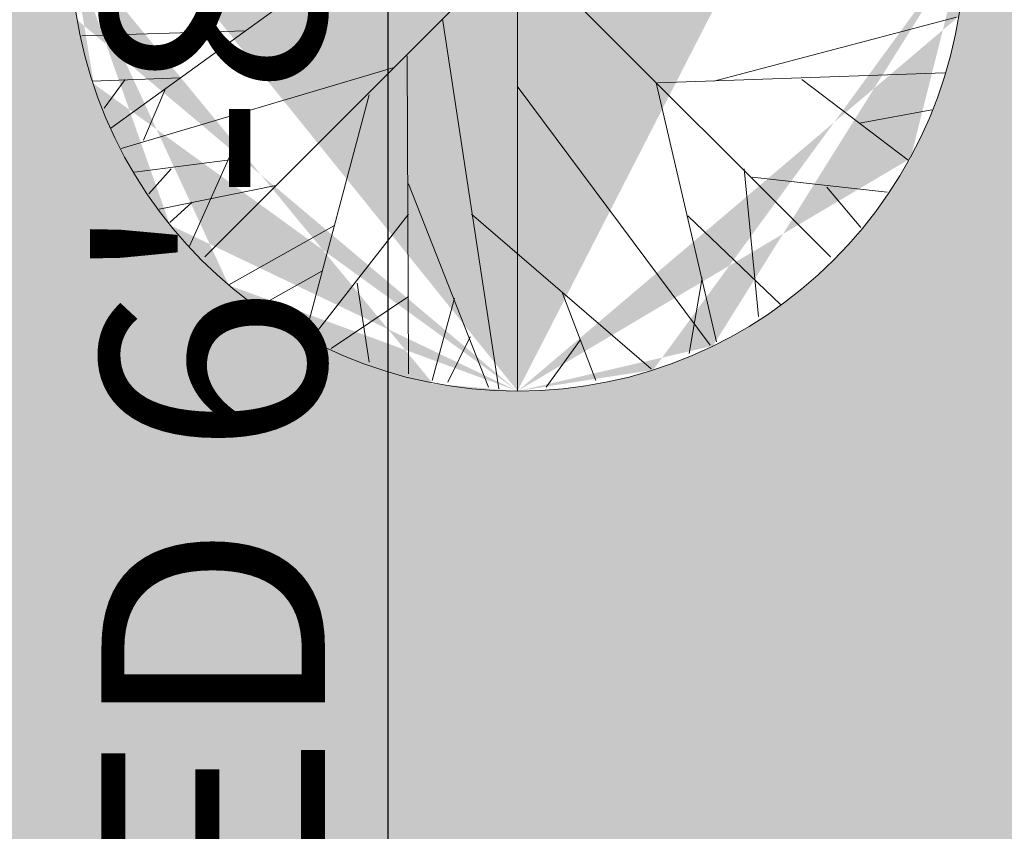
# Model space of a CAD drawing. Units: inches. Extents: x 459864 to 460310, y 324185 to 324787.
# Tile 59 of 112: x 460127 to 460154, y 324239 to 324260. Entities that reach past the tile are written whole.
import ezdxf

# ---------------------------------------------------------------- set-up
doc = ezdxf.new("R2010")
doc.units = ezdxf.units.IN
for name, color, linetype, lineweight in [('A-ANNO-DIMS', 2, 'Continuous', 18), ('L-PLNT', 3, 'Continuous', 13), ('L-SITE-PATT', 252, 'Continuous', 13)]:
    doc.layers.add(name, color=color, linetype=linetype, lineweight=lineweight)
doc.styles.get("Standard").update_dxf_attribs({"font": 'arial.ttf'})
doc.dimstyles.new('ISO-25', dxfattribs={"dimtxt": 6, "dimasz": 2.5, "dimexe": 1.25, "dimexo": 0.625, "dimtad": 1, "dimdec": 1, "dimlunit": 3, "dimtxsty": 'Standard', "dimcen": 2.5, "dimadec": 0, "dimazin": 0, "dimtfac": 1, "dimtdec": 1, "dimtmove": 0, "dimatfit": 3, "dimfxl": 1, "dimarcsym": 0})

# ---------------------------------------------------------------- blocks, each defined once
blk = doc.blocks.new('Tree - deciduous plan')
for p, q in [((0, 59.9996), (0, -60)), ((42, 42), (-42, -42)), ((42, -42), (-42, 42)), ((-54.6162, -24.7335), (-20.2853, 0.0941)), ((-10.074, -10.0627), (-2.5036, -59.7178)), ((26.3697, -18.4138), (58.9401, -9.8369)), ((-58.4895, -12.3197), (-36.4825, -11.6426)), ((-14.8275, -15.0282), (-14.6515, -57.6865)), ((-53.2078, -27.442), (-16.7641, -16.6081)), ((-57.081, -18.4138), (-45.2853, -17.9624)), ((-52.6797, -18.188), (-55.4966, -22.0251)), ((18.7992, -18.6394), (57.3556, -17.2853)), ((38.1654, -18.188), (52.426, -29.0219)), ((-47.2219, -19.3166), (-50.2148, -26.3135)), ((-0.0388, -19.0909), (25.8415, -53.8495)), ((18.6232, -18.6394), (26.7218, -53.3981)), ((-19.9331, -20.2194), (-28.5599, -52.721)), ((45.9119, -24.0564), (55.595, -22.2508)), ((-35.9543, -22.4765), (-44.0529, -40.5329)), ((-38.9472, -29.0219), (-51.4472, -30.6018)), ((-46.5177, -30.1504), (-49.5106, -33.536)), ((30.419, -30.1504), (32.3556, -50.0125)), ((31.4753, -31.279), (49.6091, -33.3103)), ((-32.4331, -32.4075), (-48.1021, -35.5674)), ((-14.6515, -32.1818), (-3.912, -59.4922)), ((41.5105, -32.6332), (46.088, -38.0501)), ((-43.7008, -34.6645), (-46.6937, -37.373)), ((-14.6515, -36.2445), (-27.6797, -52.9467)), ((-6.2008, -36.2445), (17.919, -57.0094)), ((22.8485, -36.4702), (35.3485, -48.4326)), ((-24.6867, -37.8244), (-38.7712, -45.7241)), ((-26.2712, -43.9185), (-34.7219, -48.6583)), ((24.7852, -44.8213), (23.0246, -54.978)), ((-21.5177, -45.4984), (-19.9331, -56.1065)), ((-14.6515, -47.3041), (-25.0388, -54.3009)), ((-8.4895, -47.5298), (-11.4825, -58.5893)), ((5.9471, -46.6269), (10.5246, -58.5893)), ((-6.3768, -52.721), (-9.3698, -58.815)), ((8.4119, -53.1724), (3.8344, -59.4922))]:
    blk.add_line(p, q)
blk.add_circle((0, 0), 60)
blk = doc.blocks.new('*D28')
at = {"layer": 'A-ANNO-DIMS', "color": 0, "lineweight": -2, "transparency": 16777216}
for p, q in [((460148.65, 324370.7), (460136.025, 324370.7)), ((460137.275, 324368.2), (460137.275, 324293.2)), ((460148.65, 324290.7), (460136.025, 324290.7)), ((460137.275, 324290.7), (460137.275, 324198.69))]:
    blk.add_line(p, q, dxfattribs=at)
at = {"layer": 'A-ANNO-DIMS', "color": 0, "transparency": 16777216}
for points in [[(460136.858, 324368.2), (460137.692, 324368.2), (460137.275, 324370.7)], [(460136.858, 324293.2), (460137.692, 324293.2), (460137.275, 324290.7)]]:
    blk.add_solid(points, dxfattribs=at)
at = {"layer": 'Defpoints', "color": 0, "transparency": 16777216}
for p in [(460149.275, 324370.7), (460137.275, 324290.7), (460149.275, 324290.7)]:
    blk.add_point(p, dxfattribs=at)
at = {"layer": 'A-ANNO-DIMS', "color": 0, "transparency": 16777216, "insert": (460133.363, 324243.445), "char_height": 6, "attachment_point": 5, "rotation": 90}
blk.add_mtext('QUEEN BED 6\'-8" TYP.', dxfattribs=at)

msp = doc.modelspace()

# ---------------------------------------------------------------- hatches: boundary and pattern name
at = {"layer": 'L-SITE-PATT'}
h = msp.add_hatch(dxfattribs=at)
h.set_pattern_fill('DOTS', color=256)
h.paths.add_polyline_path([(460269.804, 324283.483), (460247.115, 324283.483), (460121.929, 324283.483), (460121.929, 324252.473), (460117.429, 324252.473), (460110.124, 324252.473), (460110.124, 324243.287), (460080.83, 324243.287), (460080.83, 324252.473), (460061.115, 324252.473), (460061.115, 324251.882), (460077.909, 324251.882), (460077.909, 324199.483), (460080.83, 324199.483), (460080.83, 324207.553), (460110.124, 324207.553), (460110.124, 324199.483), (460110.813, 324199.483), (460262.115, 324199.483), (460269.804, 324199.483)], flags=17)
edge = h.paths.add_edge_path(flags=0)
edge.add_ellipse((460222.59, 324263.813), major_axis=(-8.485, 8.485), ratio=1, start_angle=405, end_angle=495, ccw=False)
edge.add_line((460214.821, 324254.66), (460214.832, 324254.666))
edge.add_ellipse((460222.59, 324263.813), major_axis=(-8.485, 8.485), ratio=1, start_angle=405, end_angle=495, ccw=False)
edge.add_line((460210.759, 324261.781), (460210.768, 324261.787))
edge.add_ellipse((460222.59, 324263.813), major_axis=(-8.485, 8.485), ratio=1, start_angle=405, end_angle=495, ccw=False)
edge.add_ellipse((460222.59, 324263.813), major_axis=(-8.485, 8.485), ratio=1, start_angle=392.754, end_angle=405, ccw=False)
edge.add_ellipse((460222.59, 324263.813), major_axis=(-8.485, 8.485), ratio=1, start_angle=380.9347, end_angle=392.754, ccw=False)
edge.add_line((460211.337, 324267.985), (460211.34, 324267.985))
edge.add_ellipse((460222.59, 324263.813), major_axis=(-8.485, 8.485), ratio=1, start_angle=380.9347, end_angle=392.754, ccw=False)
edge.add_ellipse((460222.59, 324263.813), major_axis=(-8.485, 8.485), ratio=1, start_angle=347.9015, end_angle=380.9347, ccw=False)
edge.add_ellipse((460222.59, 324263.813), major_axis=(-8.485, 8.485), ratio=1, start_angle=327.0619, end_angle=347.9015, ccw=False)
edge.add_ellipse((460222.59, 324263.813), major_axis=(-8.485, 8.485), ratio=1, start_angle=278.3246, end_angle=327.0619, ccw=False)
edge.add_line((460225.158, 324275.536), (460225.158, 324275.535))
edge.add_ellipse((460222.59, 324263.813), major_axis=(-8.485, 8.485), ratio=1, start_angle=278.3246, end_angle=327.0619, ccw=False)
edge.add_ellipse((460222.59, 324263.813), major_axis=(-8.485, 8.485), ratio=1, start_angle=260.6436, end_angle=278.3246, ccw=False)
edge.add_ellipse((460222.59, 324263.813), major_axis=(-8.485, 8.485), ratio=1, start_angle=225, end_angle=260.6436, ccw=False)
edge.add_line((460234.509, 324265.243), (460234.501, 324265.239))
edge.add_ellipse((460222.59, 324263.813), major_axis=(-8.485, 8.485), ratio=1, start_angle=225, end_angle=260.6436, ccw=False)
edge.add_ellipse((460222.59, 324263.813), major_axis=(-8.485, 8.485), ratio=1, start_angle=495, end_angle=585, ccw=False)
edge.add_line((460234.437, 324261.861), (460234.424, 324261.858))
edge.add_ellipse((460222.59, 324263.813), major_axis=(-8.485, 8.485), ratio=1, start_angle=495, end_angle=585, ccw=False)
edge.add_line((460227.95, 324253.067), (460227.946, 324253.083))
edge.add_ellipse((460222.59, 324263.813), major_axis=(-8.485, 8.485), ratio=1, start_angle=495, end_angle=585, ccw=False)
edge.add_line((460226.223, 324252.369), (460226.211, 324252.38))
edge.add_ellipse((460222.59, 324263.813), major_axis=(-8.485, 8.485), ratio=1, start_angle=495, end_angle=585, ccw=False)
h.paths.add_polyline_path([(460219.651, 324254.347), (460218.461, 324253.545), (460218.275, 324254.789), (460219.642, 324256.542), (460219.625, 324260.848), (460216.11, 324257.333), (460214.35, 324256.978), (460215.416, 324259.356), (460212.524, 324258.496), (460213.137, 324259.93), (460218.507, 324263.813), (460222.59, 324263.813), (460222.59, 324267.807), (460218.176, 324272.212), (460219.026, 324274.639), (460222.59, 324272.811), (460222.59, 324275.423), (460223.057, 324274.825), (460222.675, 324273.492), (460225.912, 324267.135), (460219.625, 324260.848)], flags=0)
edge = h.paths.add_edge_path(flags=0)
edge.add_ellipse((460194.576, 324264.046), major_axis=(-8.485, 8.485), ratio=1, start_angle=495, end_angle=585, ccw=False)
edge.add_line((460199.936, 324253.3), (460199.932, 324253.316))
edge.add_ellipse((460194.576, 324264.046), major_axis=(-8.485, 8.485), ratio=1, start_angle=495, end_angle=585, ccw=False)
edge.add_line((460198.208, 324252.603), (460198.196, 324252.613))
edge.add_ellipse((460194.576, 324264.046), major_axis=(-8.485, 8.485), ratio=1, start_angle=495, end_angle=585, ccw=False)
edge.add_ellipse((460194.576, 324264.046), major_axis=(-8.485, 8.485), ratio=1, start_angle=405, end_angle=495, ccw=False)
edge.add_line((460186.806, 324254.893), (460186.817, 324254.899))
edge.add_ellipse((460194.576, 324264.046), major_axis=(-8.485, 8.485), ratio=1, start_angle=405, end_angle=495, ccw=False)
edge.add_line((460182.744, 324262.014), (460182.753, 324262.02))
edge.add_ellipse((460194.576, 324264.046), major_axis=(-8.485, 8.485), ratio=1, start_angle=405, end_angle=495, ccw=False)
edge.add_ellipse((460194.576, 324264.046), major_axis=(-8.485, 8.485), ratio=1, start_angle=392.754, end_angle=405, ccw=False)
edge.add_ellipse((460194.576, 324264.046), major_axis=(-8.485, 8.485), ratio=1, start_angle=380.9347, end_angle=392.754, ccw=False)
edge.add_line((460183.323, 324268.218), (460183.326, 324268.218))
edge.add_ellipse((460194.576, 324264.046), major_axis=(-8.485, 8.485), ratio=1, start_angle=380.9347, end_angle=392.754, ccw=False)
edge.add_ellipse((460194.576, 324264.046), major_axis=(-8.485, 8.485), ratio=1, start_angle=347.9015, end_angle=380.9347, ccw=False)
edge.add_ellipse((460194.576, 324264.046), major_axis=(-8.485, 8.485), ratio=1, start_angle=327.0619, end_angle=347.9015, ccw=False)
edge.add_ellipse((460194.576, 324264.046), major_axis=(-8.485, 8.485), ratio=1, start_angle=278.3246, end_angle=327.0619, ccw=False)
edge.add_line((460197.144, 324275.769), (460197.143, 324275.768))
edge.add_ellipse((460194.576, 324264.046), major_axis=(-8.485, 8.485), ratio=1, start_angle=278.3246, end_angle=327.0619, ccw=False)
edge.add_ellipse((460194.576, 324264.046), major_axis=(-8.485, 8.485), ratio=1, start_angle=260.6436, end_angle=278.3246, ccw=False)
edge.add_ellipse((460194.576, 324264.046), major_axis=(-8.485, 8.485), ratio=1, start_angle=225, end_angle=260.6436, ccw=False)
edge.add_line((460206.494, 324265.476), (460206.487, 324265.473))
edge.add_ellipse((460194.576, 324264.046), major_axis=(-8.485, 8.485), ratio=1, start_angle=225, end_angle=260.6436, ccw=False)
edge.add_ellipse((460194.576, 324264.046), major_axis=(-8.485, 8.485), ratio=1, start_angle=495, end_angle=585, ccw=False)
edge.add_line((460206.422, 324262.094), (460206.409, 324262.091))
h.paths.add_polyline_path([(460191.61, 324261.081), (460191.637, 324254.58), (460190.447, 324253.778), (460190.261, 324255.023), (460191.628, 324256.775), (460191.61, 324261.081), (460188.096, 324257.566), (460186.335, 324257.211), (460187.402, 324259.589), (460184.509, 324258.729), (460185.123, 324260.163), (460190.493, 324264.046), (460194.576, 324264.046), (460194.576, 324268.04), (460190.161, 324272.446), (460191.011, 324274.872), (460194.576, 324273.044), (460194.576, 324275.657), (460195.043, 324275.058), (460194.661, 324273.725), (460197.897, 324267.368)], flags=0)
edge = h.paths.add_edge_path(flags=0)
edge.add_ellipse((460252.912, 324263.578), major_axis=(-8.485, 8.485), ratio=1, start_angle=405, end_angle=495, ccw=False)
edge.add_line((460241.081, 324261.545), (460241.089, 324261.551))
edge.add_ellipse((460252.912, 324263.578), major_axis=(-8.485, 8.485), ratio=1, start_angle=405, end_angle=495, ccw=False)
edge.add_ellipse((460252.912, 324263.578), major_axis=(-8.485, 8.485), ratio=1, start_angle=392.754, end_angle=405, ccw=False)
edge.add_ellipse((460252.912, 324263.578), major_axis=(-8.485, 8.485), ratio=1, start_angle=380.9347, end_angle=392.754, ccw=False)
edge.add_line((460241.659, 324267.749), (460241.662, 324267.749))
edge.add_ellipse((460252.912, 324263.578), major_axis=(-8.485, 8.485), ratio=1, start_angle=380.9347, end_angle=392.754, ccw=False)
edge.add_ellipse((460252.912, 324263.578), major_axis=(-8.485, 8.485), ratio=1, start_angle=347.9015, end_angle=380.9347, ccw=False)
edge.add_ellipse((460252.912, 324263.578), major_axis=(-8.485, 8.485), ratio=1, start_angle=327.0619, end_angle=347.9015, ccw=False)
edge.add_ellipse((460252.912, 324263.578), major_axis=(-8.485, 8.485), ratio=1, start_angle=278.3246, end_angle=327.0619, ccw=False)
edge.add_line((460255.48, 324275.3), (460255.479, 324275.299))
edge.add_ellipse((460252.912, 324263.578), major_axis=(-8.485, 8.485), ratio=1, start_angle=278.3246, end_angle=327.0619, ccw=False)
edge.add_ellipse((460252.912, 324263.578), major_axis=(-8.485, 8.485), ratio=1, start_angle=260.6436, end_angle=278.3246, ccw=False)
edge.add_ellipse((460252.912, 324263.578), major_axis=(-8.485, 8.485), ratio=1, start_angle=225, end_angle=260.6436, ccw=False)
edge.add_line((460264.83, 324265.007), (460264.823, 324265.004))
edge.add_ellipse((460252.912, 324263.578), major_axis=(-8.485, 8.485), ratio=1, start_angle=225, end_angle=260.6436, ccw=False)
edge.add_ellipse((460252.912, 324263.578), major_axis=(-8.485, 8.485), ratio=1, start_angle=495, end_angle=585, ccw=False)
edge.add_line((460264.758, 324261.626), (460264.745, 324261.622))
edge.add_ellipse((460252.912, 324263.578), major_axis=(-8.485, 8.485), ratio=1, start_angle=495, end_angle=585, ccw=False)
edge.add_line((460258.272, 324252.832), (460258.268, 324252.848))
edge.add_ellipse((460252.912, 324263.578), major_axis=(-8.485, 8.485), ratio=1, start_angle=495, end_angle=585, ccw=False)
edge.add_line((460256.545, 324252.134), (460256.533, 324252.144))
edge.add_ellipse((460252.912, 324263.578), major_axis=(-8.485, 8.485), ratio=1, start_angle=495, end_angle=585, ccw=False)
edge.add_ellipse((460252.912, 324263.578), major_axis=(-8.485, 8.485), ratio=1, start_angle=405, end_angle=495, ccw=False)
edge.add_line((460245.143, 324254.424), (460245.153, 324254.43))
h.paths.add_polyline_path([(460244.672, 324256.742), (460245.738, 324259.12), (460242.846, 324258.26), (460243.459, 324259.694), (460248.829, 324263.578), (460252.912, 324263.578), (460252.912, 324267.571), (460248.497, 324271.977), (460249.348, 324274.403), (460252.912, 324272.576), (460252.912, 324275.188), (460253.379, 324274.589), (460252.997, 324273.257), (460256.233, 324266.899), (460249.946, 324260.612), (460249.973, 324254.111), (460248.783, 324253.309), (460248.597, 324254.554), (460249.964, 324256.306), (460249.946, 324260.612), (460246.432, 324257.097)], flags=0)
edge = h.paths.add_edge_path(flags=0)
edge.add_ellipse((460167.439, 324262.833), major_axis=(-8.485, 8.485), ratio=1, start_angle=495, end_angle=585, ccw=False)
edge.add_line((460172.799, 324252.087), (460172.795, 324252.103))
edge.add_ellipse((460167.439, 324262.833), major_axis=(-8.485, 8.485), ratio=1, start_angle=495, end_angle=585, ccw=False)
edge.add_line((460171.071, 324251.389), (460171.059, 324251.399))
edge.add_ellipse((460167.439, 324262.833), major_axis=(-8.485, 8.485), ratio=1, start_angle=495, end_angle=585, ccw=False)
edge.add_ellipse((460167.439, 324262.833), major_axis=(-8.485, 8.485), ratio=1, start_angle=405, end_angle=495, ccw=False)
edge.add_line((460159.669, 324253.679), (460159.68, 324253.685))
edge.add_ellipse((460167.439, 324262.833), major_axis=(-8.485, 8.485), ratio=1, start_angle=405, end_angle=495, ccw=False)
edge.add_line((460155.607, 324260.8), (460155.616, 324260.806))
edge.add_ellipse((460167.439, 324262.833), major_axis=(-8.485, 8.485), ratio=1, start_angle=405, end_angle=495, ccw=False)
edge.add_ellipse((460167.439, 324262.833), major_axis=(-8.485, 8.485), ratio=1, start_angle=392.754, end_angle=405, ccw=False)
edge.add_ellipse((460167.439, 324262.833), major_axis=(-8.485, 8.485), ratio=1, start_angle=380.9347, end_angle=392.754, ccw=False)
edge.add_line((460156.185, 324267.005), (460156.189, 324267.005))
edge.add_ellipse((460167.439, 324262.833), major_axis=(-8.485, 8.485), ratio=1, start_angle=380.9347, end_angle=392.754, ccw=False)
edge.add_ellipse((460167.439, 324262.833), major_axis=(-8.485, 8.485), ratio=1, start_angle=347.9015, end_angle=380.9347, ccw=False)
edge.add_ellipse((460167.439, 324262.833), major_axis=(-8.485, 8.485), ratio=1, start_angle=327.0619, end_angle=347.9015, ccw=False)
edge.add_ellipse((460167.439, 324262.833), major_axis=(-8.485, 8.485), ratio=1, start_angle=278.3246, end_angle=327.0619, ccw=False)
edge.add_line((460170.007, 324274.556), (460170.006, 324274.554))
edge.add_ellipse((460167.439, 324262.833), major_axis=(-8.485, 8.485), ratio=1, start_angle=278.3246, end_angle=327.0619, ccw=False)
edge.add_ellipse((460167.439, 324262.833), major_axis=(-8.485, 8.485), ratio=1, start_angle=260.6436, end_angle=278.3246, ccw=False)
edge.add_ellipse((460167.439, 324262.833), major_axis=(-8.485, 8.485), ratio=1, start_angle=225, end_angle=260.6436, ccw=False)
edge.add_line((460179.357, 324264.262), (460179.35, 324264.259))
edge.add_ellipse((460167.439, 324262.833), major_axis=(-8.485, 8.485), ratio=1, start_angle=225, end_angle=260.6436, ccw=False)
edge.add_ellipse((460167.439, 324262.833), major_axis=(-8.485, 8.485), ratio=1, start_angle=495, end_angle=585, ccw=False)
edge.add_line((460179.285, 324260.881), (460179.272, 324260.877))
h.paths.add_polyline_path([(460164.473, 324259.867), (460164.5, 324253.366), (460163.31, 324252.565), (460163.124, 324253.809), (460164.491, 324255.561), (460164.473, 324259.867), (460160.958, 324256.353), (460159.198, 324255.998), (460160.265, 324258.375), (460157.372, 324257.515), (460157.986, 324258.949), (460163.356, 324262.833), (460167.439, 324262.833), (460167.439, 324266.826), (460163.024, 324271.232), (460163.874, 324273.659), (460167.439, 324271.831), (460167.439, 324274.443), (460167.905, 324273.844), (460167.524, 324272.512), (460170.76, 324266.154)], flags=0)
edge = h.paths.add_edge_path(flags=0)
edge.add_ellipse((460140.758, 324262.37), major_axis=(-8.485, 8.485), ratio=1, start_angle=495, end_angle=585, ccw=False)
edge.add_line((460146.118, 324251.624), (460146.114, 324251.639))
edge.add_ellipse((460140.758, 324262.37), major_axis=(-8.485, 8.485), ratio=1, start_angle=495, end_angle=585, ccw=False)
edge.add_line((460144.391, 324250.926), (460144.379, 324250.936))
edge.add_ellipse((460140.758, 324262.37), major_axis=(-8.485, 8.485), ratio=1, start_angle=495, end_angle=585, ccw=False)
edge.add_ellipse((460140.758, 324262.37), major_axis=(-8.485, 8.485), ratio=1, start_angle=405, end_angle=495, ccw=False)
edge.add_line((460132.989, 324253.216), (460132.999, 324253.222))
edge.add_ellipse((460140.758, 324262.37), major_axis=(-8.485, 8.485), ratio=1, start_angle=405, end_angle=495, ccw=False)
edge.add_line((460128.927, 324260.337), (460128.935, 324260.343))
edge.add_ellipse((460140.758, 324262.37), major_axis=(-8.485, 8.485), ratio=1, start_angle=405, end_angle=495, ccw=False)
edge.add_ellipse((460140.758, 324262.37), major_axis=(-8.485, 8.485), ratio=1, start_angle=392.754, end_angle=405, ccw=False)
edge.add_ellipse((460140.758, 324262.37), major_axis=(-8.485, 8.485), ratio=1, start_angle=380.9347, end_angle=392.754, ccw=False)
edge.add_line((460129.505, 324266.541), (460129.508, 324266.541))
edge.add_ellipse((460140.758, 324262.37), major_axis=(-8.485, 8.485), ratio=1, start_angle=380.9347, end_angle=392.754, ccw=False)
edge.add_ellipse((460140.758, 324262.37), major_axis=(-8.485, 8.485), ratio=1, start_angle=347.9015, end_angle=380.9347, ccw=False)
edge.add_ellipse((460140.758, 324262.37), major_axis=(-8.485, 8.485), ratio=1, start_angle=327.0619, end_angle=347.9015, ccw=False)
edge.add_ellipse((460140.758, 324262.37), major_axis=(-8.485, 8.485), ratio=1, start_angle=278.3246, end_angle=327.0619, ccw=False)
edge.add_line((460143.326, 324274.092), (460143.325, 324274.091))
edge.add_ellipse((460140.758, 324262.37), major_axis=(-8.485, 8.485), ratio=1, start_angle=278.3246, end_angle=327.0619, ccw=False)
edge.add_ellipse((460140.758, 324262.37), major_axis=(-8.485, 8.485), ratio=1, start_angle=260.6436, end_angle=278.3246, ccw=False)
edge.add_ellipse((460140.758, 324262.37), major_axis=(-8.485, 8.485), ratio=1, start_angle=225, end_angle=260.6436, ccw=False)
edge.add_line((460152.677, 324263.799), (460152.669, 324263.796))
edge.add_ellipse((460140.758, 324262.37), major_axis=(-8.485, 8.485), ratio=1, start_angle=225, end_angle=260.6436, ccw=False)
edge.add_ellipse((460140.758, 324262.37), major_axis=(-8.485, 8.485), ratio=1, start_angle=495, end_angle=585, ccw=False)
edge.add_line((460152.604, 324260.418), (460152.592, 324260.414))
h.paths.add_polyline_path([(460137.792, 324259.404), (460137.819, 324252.903), (460136.629, 324252.101), (460136.443, 324253.346), (460137.81, 324255.098), (460137.792, 324259.404), (460134.278, 324255.889), (460132.518, 324255.534), (460133.584, 324257.912), (460130.692, 324257.052), (460131.305, 324258.486), (460136.675, 324262.37), (460140.758, 324262.37), (460140.758, 324266.363), (460136.343, 324270.769), (460137.194, 324273.195), (460140.758, 324271.367), (460140.758, 324273.98), (460141.225, 324273.381), (460140.843, 324272.049), (460144.079, 324265.691)], flags=0)
h.paths.add_polyline_path([(460110.124, 324227.414), (460080.83, 324227.414), (460080.83, 324235.484), (460110.124, 324235.484)], flags=16)
h.paths.add_polyline_path([(460110.124, 324220.797), (460110.124, 324212.727), (460080.83, 324212.727), (460080.83, 324220.797)], flags=16)
h.paths.add_polyline_path([(460269.804, 324283.483), (460247.115, 324283.483), (460121.929, 324283.483), (460121.929, 324252.473), (460117.429, 324252.473), (460110.124, 324252.473), (460110.124, 324243.287), (460080.83, 324243.287), (460080.83, 324252.473), (460061.115, 324252.473), (460061.115, 324251.882), (460077.909, 324251.882), (460077.909, 324199.483), (460080.83, 324199.483), (460080.83, 324207.553), (460110.124, 324207.553), (460110.124, 324199.483), (460262.115, 324199.483), (460269.804, 324199.483)], flags=17)
h.paths.add_polyline_path([(460219.651, 324254.347), (460218.461, 324253.545), (460218.275, 324254.789), (460219.642, 324256.542), (460219.625, 324260.848), (460216.11, 324257.333), (460214.35, 324256.978), (460215.416, 324259.356), (460212.524, 324258.496), (460213.137, 324259.93), (460218.507, 324263.813), (460222.59, 324263.813), (460220.18, 324266.223), (460215.461, 324265.308), (460211.835, 324266.137), (460216.247, 324267.985), (460218.418, 324267.985), (460222.59, 324263.813), (460222.59, 324267.807), (460218.176, 324272.212), (460219.026, 324274.639), (460222.59, 324272.811), (460222.59, 324275.423), (460223.057, 324274.825), (460222.675, 324273.492), (460225.912, 324267.135), (460222.59, 324263.813), (460231.383, 324263.813), (460228.485, 324262.488), (460224.425, 324261.978), (460228.68, 324257.724), (460228.966, 324254.791), (460227.142, 324256.537), (460227.542, 324254.819), (460227.333, 324253.614), (460222.59, 324259.985), (460222.59, 324255.497), (460221.377, 324256.541), (460220.576, 324261.799), (460219.625, 324260.848)], flags=0)
h.paths.add_polyline_path([(460199.127, 324256.77), (460199.528, 324255.052), (460199.319, 324253.848), (460194.576, 324260.218), (460194.576, 324255.73), (460193.363, 324256.774), (460192.561, 324262.032), (460191.61, 324261.081), (460191.637, 324254.58), (460190.447, 324253.778), (460190.261, 324255.023), (460191.628, 324256.775), (460191.61, 324261.081), (460188.096, 324257.566), (460186.335, 324257.211), (460187.402, 324259.589), (460184.509, 324258.729), (460185.123, 324260.163), (460190.493, 324264.046), (460194.576, 324264.046), (460192.166, 324266.456), (460187.446, 324265.541), (460183.82, 324266.37), (460188.232, 324268.218), (460190.404, 324268.218), (460194.576, 324264.046), (460194.576, 324268.04), (460190.161, 324272.446), (460191.011, 324274.872), (460194.576, 324273.044), (460194.576, 324275.657), (460195.043, 324275.058), (460194.661, 324273.725), (460197.897, 324267.368), (460194.576, 324264.046), (460203.368, 324264.046), (460200.47, 324262.721), (460196.411, 324262.212), (460200.665, 324257.957), (460200.951, 324255.024)], flags=0)
h.paths.add_polyline_path([(460244.672, 324256.742), (460245.738, 324259.12), (460242.846, 324258.26), (460243.459, 324259.694), (460248.829, 324263.578), (460252.912, 324263.578), (460250.502, 324265.987), (460245.783, 324265.072), (460242.156, 324265.901), (460246.568, 324267.749), (460248.74, 324267.749), (460252.912, 324263.578), (460252.912, 324267.571), (460248.497, 324271.977), (460249.348, 324274.403), (460252.912, 324272.576), (460252.912, 324275.188), (460253.379, 324274.589), (460252.997, 324273.257), (460256.233, 324266.899), (460252.912, 324263.578), (460261.705, 324263.578), (460258.806, 324262.252), (460254.747, 324261.743), (460259.002, 324257.488), (460259.288, 324254.555), (460257.463, 324256.301), (460257.864, 324254.583), (460257.655, 324253.379), (460252.912, 324259.749), (460252.912, 324255.261), (460251.699, 324256.305), (460250.897, 324261.563), (460249.946, 324260.612), (460249.973, 324254.111), (460248.783, 324253.309), (460248.597, 324254.554), (460249.964, 324256.306), (460249.946, 324260.612), (460246.432, 324257.097)], flags=0)
h.paths.add_polyline_path([(460173.528, 324256.743), (460173.814, 324253.811), (460171.99, 324255.556), (460172.39, 324253.838), (460172.182, 324252.634), (460167.439, 324259.004), (460167.439, 324254.516), (460166.226, 324255.56), (460165.424, 324260.818), (460164.473, 324259.867), (460164.5, 324253.366), (460163.31, 324252.565), (460163.124, 324253.809), (460164.491, 324255.561), (460164.473, 324259.867), (460160.958, 324256.353), (460159.198, 324255.998), (460160.265, 324258.375), (460157.372, 324257.515), (460157.986, 324258.949), (460163.356, 324262.833), (460167.439, 324262.833), (460165.029, 324265.243), (460160.309, 324264.327), (460156.683, 324265.156), (460161.095, 324267.005), (460163.267, 324267.005), (460167.439, 324262.833), (460167.439, 324266.826), (460163.024, 324271.232), (460163.874, 324273.659), (460167.439, 324271.831), (460167.439, 324274.443), (460167.905, 324273.844), (460167.524, 324272.512), (460170.76, 324266.154), (460167.439, 324262.833), (460176.231, 324262.833), (460173.333, 324261.507), (460169.274, 324260.998)], flags=0)
h.paths.add_polyline_path([(460146.848, 324256.28), (460147.134, 324253.347), (460145.31, 324255.093), (460145.71, 324253.375), (460145.501, 324252.171), (460140.758, 324258.541), (460140.758, 324254.053), (460139.545, 324255.097), (460138.744, 324260.355), (460137.792, 324259.404), (460137.819, 324252.903), (460136.629, 324252.101), (460136.443, 324253.346), (460137.81, 324255.098), (460137.792, 324259.404), (460134.278, 324255.889), (460132.518, 324255.534), (460133.584, 324257.912), (460130.692, 324257.052), (460131.305, 324258.486), (460136.675, 324262.37), (460140.758, 324262.37), (460138.348, 324264.779), (460133.629, 324263.864), (460130.002, 324264.693), (460134.414, 324266.541), (460136.586, 324266.541), (460140.758, 324262.37), (460140.758, 324266.363), (460136.343, 324270.769), (460137.194, 324273.195), (460140.758, 324271.367), (460140.758, 324273.98), (460141.225, 324273.381), (460140.843, 324272.049), (460144.079, 324265.691), (460140.758, 324262.37), (460149.551, 324262.37), (460146.653, 324261.044), (460142.593, 324260.535)], flags=0)
edge = h.paths.add_edge_path()
edge.add_line((460269.804, 324272.549), (460260.881, 324272.549))
edge.add_ellipse((460252.912, 324263.578), major_axis=(-8.485, 8.485), ratio=1, start_angle=260.6436, end_angle=273.3846, ccw=False)
edge.add_line((460262.283, 324271.092), (460262.261, 324271.091))
edge.add_ellipse((460252.912, 324263.578), major_axis=(-8.485, 8.485), ratio=1, start_angle=260.6436, end_angle=273.3846, ccw=False)
edge.add_ellipse((460252.912, 324263.578), major_axis=(-8.485, 8.485), ratio=1, start_angle=225, end_angle=260.6436, ccw=False)
edge.add_line((460263.609, 324269.063), (460263.572, 324269.058))
edge.add_ellipse((460252.912, 324263.578), major_axis=(-8.485, 8.485), ratio=1, start_angle=225, end_angle=260.6436, ccw=False)
edge.add_line((460264.615, 324266.306), (460264.585, 324266.305))
edge.add_ellipse((460252.912, 324263.578), major_axis=(-8.485, 8.485), ratio=1, start_angle=225, end_angle=260.6436, ccw=False)
edge.add_line((460264.83, 324265.007), (460264.823, 324265.004))
edge.add_ellipse((460252.912, 324263.578), major_axis=(-8.485, 8.485), ratio=1, start_angle=225, end_angle=260.6436, ccw=False)
edge.add_ellipse((460252.912, 324263.578), major_axis=(-8.485, 8.485), ratio=1, start_angle=495, end_angle=585, ccw=False)
edge.add_line((460264.758, 324261.626), (460264.745, 324261.622))
edge.add_ellipse((460252.912, 324263.578), major_axis=(-8.485, 8.485), ratio=1, start_angle=495, end_angle=585, ccw=False)
edge.add_line((460263.442, 324257.739), (460263.389, 324257.779))
edge.add_ellipse((460252.912, 324263.578), major_axis=(-8.485, 8.485), ratio=1, start_angle=495, end_angle=585, ccw=False)
edge.add_line((460258.128, 324252.744), (460258.102, 324252.779))
edge.add_ellipse((460252.912, 324263.578), major_axis=(-8.485, 8.485), ratio=1, start_angle=495, end_angle=585, ccw=False)
edge.add_line((460256.545, 324252.134), (460256.533, 324252.144))
edge.add_ellipse((460252.912, 324263.578), major_axis=(-8.485, 8.485), ratio=1, start_angle=495, end_angle=585, ccw=False)
edge.add_ellipse((460252.912, 324263.578), major_axis=(-8.485, 8.485), ratio=1, start_angle=405, end_angle=495, ccw=False)
edge.add_line((460250.594, 324251.78), (460250.605, 324251.82))
edge.add_ellipse((460252.912, 324263.578), major_axis=(-8.485, 8.485), ratio=1, start_angle=405, end_angle=495, ccw=False)
edge.add_line((460245.143, 324254.424), (460245.153, 324254.43))
edge.add_ellipse((460252.912, 324263.578), major_axis=(-8.485, 8.485), ratio=1, start_angle=405, end_angle=495, ccw=False)
edge.add_line((460243.525, 324256.059), (460243.56, 324256.091))
edge.add_ellipse((460252.912, 324263.578), major_axis=(-8.485, 8.485), ratio=1, start_angle=405, end_angle=495, ccw=False)
edge.add_line((460241.44, 324259.893), (460241.522, 324259.896))
edge.add_ellipse((460252.912, 324263.578), major_axis=(-8.485, 8.485), ratio=1, start_angle=405, end_angle=495, ccw=False)
edge.add_line((460241.081, 324261.545), (460241.089, 324261.551))
edge.add_ellipse((460252.912, 324263.578), major_axis=(-8.485, 8.485), ratio=1, start_angle=405, end_angle=495, ccw=False)
edge.add_ellipse((460252.912, 324263.578), major_axis=(-8.485, 8.485), ratio=1, start_angle=392.754, end_angle=405, ccw=False)
edge.add_line((460241.05, 324265.438), (460241.063, 324265.443))
edge.add_ellipse((460252.912, 324263.578), major_axis=(-8.485, 8.485), ratio=1, start_angle=392.754, end_angle=405, ccw=False)
edge.add_ellipse((460252.912, 324263.578), major_axis=(-8.485, 8.485), ratio=1, start_angle=380.9347, end_angle=392.754, ccw=False)
edge.add_line((460241.452, 324267.176), (460241.469, 324267.171))
edge.add_ellipse((460252.912, 324263.578), major_axis=(-8.485, 8.485), ratio=1, start_angle=380.9347, end_angle=392.754, ccw=False)
edge.add_line((460241.659, 324267.749), (460241.662, 324267.749))
edge.add_ellipse((460252.912, 324263.578), major_axis=(-8.485, 8.485), ratio=1, start_angle=380.9347, end_angle=392.754, ccw=False)
edge.add_ellipse((460252.912, 324263.578), major_axis=(-8.485, 8.485), ratio=1, start_angle=356.6154, end_angle=380.9347, ccw=False)
edge.add_line((460244.88, 324272.488), (460244.713, 324272.549))
edge.add_line((460244.713, 324272.549), (460230.817, 324272.549))
edge.add_ellipse((460222.59, 324263.813), major_axis=(-8.485, 8.485), ratio=1, start_angle=260.6436, end_angle=271.7178, ccw=False)
edge.add_ellipse((460222.59, 324263.813), major_axis=(-8.485, 8.485), ratio=1, start_angle=225, end_angle=260.6436, ccw=False)
edge.add_line((460233.287, 324269.299), (460233.25, 324269.294))
edge.add_ellipse((460222.59, 324263.813), major_axis=(-8.485, 8.485), ratio=1, start_angle=225, end_angle=260.6436, ccw=False)
edge.add_line((460234.294, 324266.541), (460234.264, 324266.541))
edge.add_ellipse((460222.59, 324263.813), major_axis=(-8.485, 8.485), ratio=1, start_angle=225, end_angle=260.6436, ccw=False)
edge.add_line((460234.509, 324265.243), (460234.501, 324265.239))
edge.add_ellipse((460222.59, 324263.813), major_axis=(-8.485, 8.485), ratio=1, start_angle=225, end_angle=260.6436, ccw=False)
edge.add_ellipse((460222.59, 324263.813), major_axis=(-8.485, 8.485), ratio=1, start_angle=495, end_angle=585, ccw=False)
edge.add_line((460234.437, 324261.861), (460234.424, 324261.858))
edge.add_ellipse((460222.59, 324263.813), major_axis=(-8.485, 8.485), ratio=1, start_angle=495, end_angle=585, ccw=False)
edge.add_line((460233.121, 324257.975), (460233.068, 324258.015))
edge.add_ellipse((460222.59, 324263.813), major_axis=(-8.485, 8.485), ratio=1, start_angle=495, end_angle=585, ccw=False)
edge.add_line((460227.806, 324252.979), (460227.78, 324253.014))
edge.add_ellipse((460222.59, 324263.813), major_axis=(-8.485, 8.485), ratio=1, start_angle=495, end_angle=585, ccw=False)
edge.add_line((460226.223, 324252.369), (460226.211, 324252.38))
edge.add_ellipse((460222.59, 324263.813), major_axis=(-8.485, 8.485), ratio=1, start_angle=495, end_angle=585, ccw=False)
edge.add_ellipse((460222.59, 324263.813), major_axis=(-8.485, 8.485), ratio=1, start_angle=405, end_angle=495, ccw=False)
edge.add_line((460220.272, 324252.016), (460220.283, 324252.055))
edge.add_ellipse((460222.59, 324263.813), major_axis=(-8.485, 8.485), ratio=1, start_angle=405, end_angle=495, ccw=False)
edge.add_line((460214.821, 324254.66), (460214.832, 324254.666))
edge.add_ellipse((460222.59, 324263.813), major_axis=(-8.485, 8.485), ratio=1, start_angle=405, end_angle=495, ccw=False)
edge.add_line((460213.203, 324256.295), (460213.239, 324256.327))
edge.add_ellipse((460222.59, 324263.813), major_axis=(-8.485, 8.485), ratio=1, start_angle=405, end_angle=495, ccw=False)
edge.add_line((460211.118, 324260.128), (460211.201, 324260.131))
edge.add_ellipse((460222.59, 324263.813), major_axis=(-8.485, 8.485), ratio=1, start_angle=405, end_angle=495, ccw=False)
edge.add_line((460210.759, 324261.781), (460210.768, 324261.787))
edge.add_ellipse((460222.59, 324263.813), major_axis=(-8.485, 8.485), ratio=1, start_angle=405, end_angle=495, ccw=False)
edge.add_ellipse((460222.59, 324263.813), major_axis=(-8.485, 8.485), ratio=1, start_angle=392.754, end_angle=405, ccw=False)
edge.add_line((460210.729, 324265.673), (460210.741, 324265.678))
edge.add_ellipse((460222.59, 324263.813), major_axis=(-8.485, 8.485), ratio=1, start_angle=392.754, end_angle=405, ccw=False)
edge.add_ellipse((460222.59, 324263.813), major_axis=(-8.485, 8.485), ratio=1, start_angle=380.9347, end_angle=392.754, ccw=False)
edge.add_line((460211.13, 324267.412), (460211.147, 324267.407))
edge.add_ellipse((460222.59, 324263.813), major_axis=(-8.485, 8.485), ratio=1, start_angle=380.9347, end_angle=392.754, ccw=False)
edge.add_line((460211.337, 324267.985), (460211.34, 324267.985))
edge.add_ellipse((460222.59, 324263.813), major_axis=(-8.485, 8.485), ratio=1, start_angle=380.9347, end_angle=392.754, ccw=False)
edge.add_ellipse((460222.59, 324263.813), major_axis=(-8.485, 8.485), ratio=1, start_angle=358.2822, end_angle=380.9347, ccw=False)
edge.add_line((460213.705, 324271.902), (460213.709, 324271.869))
edge.add_ellipse((460222.59, 324263.813), major_axis=(-8.485, 8.485), ratio=1, start_angle=358.2822, end_angle=380.9347, ccw=False)
edge.add_line((460214.363, 324272.549), (460203.078, 324272.549))
edge.add_line((460203.078, 324272.549), (460203.06, 324272.531))
edge.add_ellipse((460194.576, 324264.046), major_axis=(-8.485, 8.485), ratio=1, start_angle=260.6436, end_angle=270.1168, ccw=False)
edge.add_line((460203.957, 324271.561), (460203.921, 324271.56))
edge.add_ellipse((460194.576, 324264.046), major_axis=(-8.485, 8.485), ratio=1, start_angle=260.6436, end_angle=270.1168, ccw=False)
edge.add_ellipse((460194.576, 324264.046), major_axis=(-8.485, 8.485), ratio=1, start_angle=225, end_angle=260.6436, ccw=False)
edge.add_line((460205.272, 324269.532), (460205.235, 324269.527))
edge.add_ellipse((460194.576, 324264.046), major_axis=(-8.485, 8.485), ratio=1, start_angle=225, end_angle=260.6436, ccw=False)
edge.add_line((460206.279, 324266.774), (460206.249, 324266.774))
edge.add_ellipse((460194.576, 324264.046), major_axis=(-8.485, 8.485), ratio=1, start_angle=225, end_angle=260.6436, ccw=False)
edge.add_line((460206.494, 324265.476), (460206.487, 324265.473))
edge.add_ellipse((460194.576, 324264.046), major_axis=(-8.485, 8.485), ratio=1, start_angle=225, end_angle=260.6436, ccw=False)
edge.add_ellipse((460194.576, 324264.046), major_axis=(-8.485, 8.485), ratio=1, start_angle=495, end_angle=585, ccw=False)
edge.add_line((460206.422, 324262.094), (460206.409, 324262.091))
edge.add_ellipse((460194.576, 324264.046), major_axis=(-8.485, 8.485), ratio=1, start_angle=495, end_angle=585, ccw=False)
edge.add_line((460205.106, 324258.208), (460205.053, 324258.248))
edge.add_ellipse((460194.576, 324264.046), major_axis=(-8.485, 8.485), ratio=1, start_angle=495, end_angle=585, ccw=False)
edge.add_line((460199.792, 324253.212), (460199.766, 324253.248))
edge.add_ellipse((460194.576, 324264.046), major_axis=(-8.485, 8.485), ratio=1, start_angle=495, end_angle=585, ccw=False)
edge.add_line((460198.208, 324252.603), (460198.196, 324252.613))
edge.add_ellipse((460194.576, 324264.046), major_axis=(-8.485, 8.485), ratio=1, start_angle=495, end_angle=585, ccw=False)
edge.add_ellipse((460194.576, 324264.046), major_axis=(-8.485, 8.485), ratio=1, start_angle=405, end_angle=495, ccw=False)
edge.add_line((460192.258, 324252.249), (460192.268, 324252.289))
edge.add_ellipse((460194.576, 324264.046), major_axis=(-8.485, 8.485), ratio=1, start_angle=405, end_angle=495, ccw=False)
edge.add_line((460186.806, 324254.893), (460186.817, 324254.899))
edge.add_ellipse((460194.576, 324264.046), major_axis=(-8.485, 8.485), ratio=1, start_angle=405, end_angle=495, ccw=False)
edge.add_line((460185.188, 324256.528), (460185.224, 324256.56))
edge.add_ellipse((460194.576, 324264.046), major_axis=(-8.485, 8.485), ratio=1, start_angle=405, end_angle=495, ccw=False)
edge.add_line((460183.104, 324260.362), (460183.186, 324260.365))
edge.add_ellipse((460194.576, 324264.046), major_axis=(-8.485, 8.485), ratio=1, start_angle=405, end_angle=495, ccw=False)
edge.add_line((460182.744, 324262.014), (460182.753, 324262.02))
edge.add_ellipse((460194.576, 324264.046), major_axis=(-8.485, 8.485), ratio=1, start_angle=405, end_angle=495, ccw=False)
edge.add_ellipse((460194.576, 324264.046), major_axis=(-8.485, 8.485), ratio=1, start_angle=392.754, end_angle=405, ccw=False)
edge.add_line((460182.714, 324265.906), (460182.726, 324265.912))
edge.add_ellipse((460194.576, 324264.046), major_axis=(-8.485, 8.485), ratio=1, start_angle=392.754, end_angle=405, ccw=False)
edge.add_ellipse((460194.576, 324264.046), major_axis=(-8.485, 8.485), ratio=1, start_angle=380.9347, end_angle=392.754, ccw=False)
edge.add_line((460183.116, 324267.645), (460183.133, 324267.64))
edge.add_ellipse((460194.576, 324264.046), major_axis=(-8.485, 8.485), ratio=1, start_angle=380.9347, end_angle=392.754, ccw=False)
edge.add_line((460183.323, 324268.218), (460183.326, 324268.218))
edge.add_ellipse((460194.576, 324264.046), major_axis=(-8.485, 8.485), ratio=1, start_angle=380.9347, end_angle=392.754, ccw=False)
edge.add_ellipse((460194.576, 324264.046), major_axis=(-8.485, 8.485), ratio=1, start_angle=359.8832, end_angle=380.9347, ccw=False)
edge.add_line((460184.491, 324270.611), (460184.553, 324270.611))
edge.add_ellipse((460194.576, 324264.046), major_axis=(-8.485, 8.485), ratio=1, start_angle=359.8832, end_angle=380.9347, ccw=False)
edge.add_line((460185.346, 324271.76), (460185.379, 324271.728))
edge.add_ellipse((460194.576, 324264.046), major_axis=(-8.485, 8.485), ratio=1, start_angle=359.8832, end_angle=380.9347, ccw=False)
edge.add_line((460185.697, 324272.086), (460185.633, 324272.549))
edge.add_line((460185.633, 324272.549), (460174.683, 324272.549))
edge.add_line((460174.683, 324272.549), (460174.606, 324272.457))
edge.add_ellipse((460167.439, 324262.833), major_axis=(-8.485, 8.485), ratio=1, start_angle=260.6436, end_angle=278.3246, ccw=False)
edge.add_ellipse((460167.439, 324262.833), major_axis=(-8.485, 8.485), ratio=1, start_angle=225, end_angle=260.6436, ccw=False)
edge.add_line((460178.135, 324268.318), (460178.098, 324268.313))
edge.add_ellipse((460167.439, 324262.833), major_axis=(-8.485, 8.485), ratio=1, start_angle=225, end_angle=260.6436, ccw=False)
edge.add_line((460179.142, 324265.561), (460179.112, 324265.56))
edge.add_ellipse((460167.439, 324262.833), major_axis=(-8.485, 8.485), ratio=1, start_angle=225, end_angle=260.6436, ccw=False)
edge.add_line((460179.357, 324264.262), (460179.35, 324264.259))
edge.add_ellipse((460167.439, 324262.833), major_axis=(-8.485, 8.485), ratio=1, start_angle=225, end_angle=260.6436, ccw=False)
edge.add_ellipse((460167.439, 324262.833), major_axis=(-8.485, 8.485), ratio=1, start_angle=495, end_angle=585, ccw=False)
edge.add_line((460179.285, 324260.881), (460179.272, 324260.877))
edge.add_ellipse((460167.439, 324262.833), major_axis=(-8.485, 8.485), ratio=1, start_angle=495, end_angle=585, ccw=False)
edge.add_line((460177.969, 324256.994), (460177.916, 324257.034))
edge.add_ellipse((460167.439, 324262.833), major_axis=(-8.485, 8.485), ratio=1, start_angle=495, end_angle=585, ccw=False)
edge.add_line((460172.655, 324251.999), (460172.629, 324252.034))
edge.add_ellipse((460167.439, 324262.833), major_axis=(-8.485, 8.485), ratio=1, start_angle=495, end_angle=585, ccw=False)
edge.add_line((460171.071, 324251.389), (460171.059, 324251.399))
edge.add_ellipse((460167.439, 324262.833), major_axis=(-8.485, 8.485), ratio=1, start_angle=495, end_angle=585, ccw=False)
edge.add_ellipse((460167.439, 324262.833), major_axis=(-8.485, 8.485), ratio=1, start_angle=405, end_angle=495, ccw=False)
edge.add_line((460165.121, 324251.036), (460165.131, 324251.075))
edge.add_ellipse((460167.439, 324262.833), major_axis=(-8.485, 8.485), ratio=1, start_angle=405, end_angle=495, ccw=False)
edge.add_line((460159.669, 324253.679), (460159.68, 324253.685))
edge.add_ellipse((460167.439, 324262.833), major_axis=(-8.485, 8.485), ratio=1, start_angle=405, end_angle=495, ccw=False)
edge.add_line((460158.051, 324255.314), (460158.087, 324255.347))
edge.add_ellipse((460167.439, 324262.833), major_axis=(-8.485, 8.485), ratio=1, start_angle=405, end_angle=495, ccw=False)
edge.add_line((460155.967, 324259.148), (460156.049, 324259.151))
edge.add_ellipse((460167.439, 324262.833), major_axis=(-8.485, 8.485), ratio=1, start_angle=405, end_angle=495, ccw=False)
edge.add_line((460155.607, 324260.8), (460155.616, 324260.806))
edge.add_ellipse((460167.439, 324262.833), major_axis=(-8.485, 8.485), ratio=1, start_angle=405, end_angle=495, ccw=False)
edge.add_ellipse((460167.439, 324262.833), major_axis=(-8.485, 8.485), ratio=1, start_angle=392.754, end_angle=405, ccw=False)
edge.add_line((460155.577, 324264.693), (460155.589, 324264.698))
edge.add_ellipse((460167.439, 324262.833), major_axis=(-8.485, 8.485), ratio=1, start_angle=392.754, end_angle=405, ccw=False)
edge.add_ellipse((460167.439, 324262.833), major_axis=(-8.485, 8.485), ratio=1, start_angle=380.9347, end_angle=392.754, ccw=False)
edge.add_line((460155.979, 324266.432), (460155.996, 324266.426))
edge.add_ellipse((460167.439, 324262.833), major_axis=(-8.485, 8.485), ratio=1, start_angle=380.9347, end_angle=392.754, ccw=False)
edge.add_line((460156.185, 324267.005), (460156.189, 324267.005))
edge.add_ellipse((460167.439, 324262.833), major_axis=(-8.485, 8.485), ratio=1, start_angle=380.9347, end_angle=392.754, ccw=False)
edge.add_ellipse((460167.439, 324262.833), major_axis=(-8.485, 8.485), ratio=1, start_angle=350.9345, end_angle=380.9347, ccw=False)
edge.add_line((460157.363, 324269.397), (460157.414, 324269.397))
edge.add_ellipse((460167.439, 324262.833), major_axis=(-8.485, 8.485), ratio=1, start_angle=350.9345, end_angle=380.9347, ccw=False)
edge.add_line((460158.221, 324270.535), (460158.236, 324270.519))
edge.add_ellipse((460167.439, 324262.833), major_axis=(-8.485, 8.485), ratio=1, start_angle=350.9345, end_angle=380.9347, ccw=False)
edge.add_line((460159.379, 324271.753), (460159.419, 324271.738))
edge.add_ellipse((460167.439, 324262.833), major_axis=(-8.485, 8.485), ratio=1, start_angle=350.9345, end_angle=380.9347, ccw=False)
edge.add_line((460160.396, 324272.549), (460147.112, 324272.549))
edge.add_ellipse((460140.758, 324262.37), major_axis=(-8.485, 8.485), ratio=1, start_angle=278.3246, end_angle=283.0261, ccw=False)
edge.add_ellipse((460140.758, 324262.37), major_axis=(-8.485, 8.485), ratio=1, start_angle=260.6436, end_angle=278.3246, ccw=False)
edge.add_ellipse((460140.758, 324262.37), major_axis=(-8.485, 8.485), ratio=1, start_angle=225, end_angle=260.6436, ccw=False)
edge.add_line((460151.455, 324267.855), (460151.418, 324267.85))
edge.add_ellipse((460140.758, 324262.37), major_axis=(-8.485, 8.485), ratio=1, start_angle=225, end_angle=260.6436, ccw=False)
edge.add_line((460152.462, 324265.098), (460152.431, 324265.097))
edge.add_ellipse((460140.758, 324262.37), major_axis=(-8.485, 8.485), ratio=1, start_angle=225, end_angle=260.6436, ccw=False)
edge.add_line((460152.677, 324263.799), (460152.669, 324263.796))
edge.add_ellipse((460140.758, 324262.37), major_axis=(-8.485, 8.485), ratio=1, start_angle=225, end_angle=260.6436, ccw=False)
edge.add_ellipse((460140.758, 324262.37), major_axis=(-8.485, 8.485), ratio=1, start_angle=495, end_angle=585, ccw=False)
edge.add_line((460152.604, 324260.418), (460152.592, 324260.414))
edge.add_ellipse((460140.758, 324262.37), major_axis=(-8.485, 8.485), ratio=1, start_angle=495, end_angle=585, ccw=False)
edge.add_line((460151.288, 324256.531), (460151.235, 324256.571))
edge.add_ellipse((460140.758, 324262.37), major_axis=(-8.485, 8.485), ratio=1, start_angle=495, end_angle=585, ccw=False)
edge.add_line((460145.974, 324251.535), (460145.948, 324251.571))
edge.add_ellipse((460140.758, 324262.37), major_axis=(-8.485, 8.485), ratio=1, start_angle=495, end_angle=585, ccw=False)
edge.add_line((460144.391, 324250.926), (460144.379, 324250.936))
edge.add_ellipse((460140.758, 324262.37), major_axis=(-8.485, 8.485), ratio=1, start_angle=495, end_angle=585, ccw=False)
edge.add_ellipse((460140.758, 324262.37), major_axis=(-8.485, 8.485), ratio=1, start_angle=405, end_angle=495, ccw=False)
edge.add_line((460138.44, 324250.572), (460138.451, 324250.612))
edge.add_ellipse((460140.758, 324262.37), major_axis=(-8.485, 8.485), ratio=1, start_angle=405, end_angle=495, ccw=False)
edge.add_line((460132.989, 324253.216), (460132.999, 324253.222))
edge.add_ellipse((460140.758, 324262.37), major_axis=(-8.485, 8.485), ratio=1, start_angle=405, end_angle=495, ccw=False)
edge.add_line((460131.371, 324254.851), (460131.406, 324254.883))
edge.add_ellipse((460140.758, 324262.37), major_axis=(-8.485, 8.485), ratio=1, start_angle=405, end_angle=495, ccw=False)
edge.add_line((460129.286, 324258.685), (460129.369, 324258.688))
edge.add_ellipse((460140.758, 324262.37), major_axis=(-8.485, 8.485), ratio=1, start_angle=405, end_angle=495, ccw=False)
edge.add_line((460128.927, 324260.337), (460128.935, 324260.343))
edge.add_ellipse((460140.758, 324262.37), major_axis=(-8.485, 8.485), ratio=1, start_angle=405, end_angle=495, ccw=False)
edge.add_ellipse((460140.758, 324262.37), major_axis=(-8.485, 8.485), ratio=1, start_angle=392.754, end_angle=405, ccw=False)
edge.add_line((460128.896, 324264.23), (460128.909, 324264.235))
edge.add_ellipse((460140.758, 324262.37), major_axis=(-8.485, 8.485), ratio=1, start_angle=392.754, end_angle=405, ccw=False)
edge.add_ellipse((460140.758, 324262.37), major_axis=(-8.485, 8.485), ratio=1, start_angle=380.9347, end_angle=392.754, ccw=False)
edge.add_line((460129.298, 324265.968), (460129.315, 324265.963))
edge.add_ellipse((460140.758, 324262.37), major_axis=(-8.485, 8.485), ratio=1, start_angle=380.9347, end_angle=392.754, ccw=False)
edge.add_line((460129.505, 324266.541), (460129.508, 324266.541))
edge.add_ellipse((460140.758, 324262.37), major_axis=(-8.485, 8.485), ratio=1, start_angle=380.9347, end_angle=392.754, ccw=False)
edge.add_ellipse((460140.758, 324262.37), major_axis=(-8.485, 8.485), ratio=1, start_angle=347.9015, end_angle=380.9347, ccw=False)
edge.add_line((460130.697, 324268.934), (460130.727, 324268.934))
edge.add_ellipse((460140.758, 324262.37), major_axis=(-8.485, 8.485), ratio=1, start_angle=347.9015, end_angle=380.9347, ccw=False)
edge.add_line((460131.869, 324270.48), (460131.879, 324270.413))
edge.add_ellipse((460140.758, 324262.37), major_axis=(-8.485, 8.485), ratio=1, start_angle=347.9015, end_angle=380.9347, ccw=False)
edge.add_line((460132.734, 324271.277), (460132.705, 324271.287))
edge.add_ellipse((460140.758, 324262.37), major_axis=(-8.485, 8.485), ratio=1, start_angle=347.9015, end_angle=380.9347, ccw=False)
edge.add_line((460134.24, 324272.445), (460134.204, 324272.549))
edge.add_line((460134.204, 324272.549), (460121.929, 324272.549))
edge.add_line((460121.929, 324272.549), (460121.929, 324252.473))
edge.add_line((460121.929, 324252.473), (460117.429, 324252.473))
edge.add_line((460117.429, 324252.473), (460110.124, 324252.473))
edge.add_line((460110.124, 324252.473), (460110.124, 324243.287))
edge.add_line((460110.124, 324243.287), (460080.83, 324243.287))
edge.add_line((460080.83, 324243.287), (460080.83, 324252.473))
edge.add_line((460080.83, 324252.473), (460061.115, 324252.473))
edge.add_line((460061.115, 324252.473), (460061.115, 324251.882))
edge.add_line((460061.115, 324251.882), (460077.909, 324251.882))
edge.add_line((460077.909, 324251.882), (460077.909, 324199.483))
edge.add_line((460077.909, 324199.483), (460080.83, 324199.483))
edge.add_line((460080.83, 324199.483), (460080.83, 324207.553))
edge.add_line((460080.83, 324207.553), (460110.124, 324207.553))
edge.add_line((460110.124, 324207.553), (460110.124, 324199.483))
edge.add_line((460110.124, 324199.483), (460110.813, 324199.483))
edge.add_line((460110.813, 324199.483), (460262.115, 324199.483))
edge.add_line((460262.115, 324199.483), (460269.804, 324199.483))
edge.add_line((460269.804, 324199.483), (460269.804, 324272.549))

# ---------------------------------------------------------------- block references
at = {"layer": 'L-PLNT', "xscale": 0.2, "yscale": 0.2}
msp.add_blockref('Tree - deciduous plan', (460140.758, 324262.37), dxfattribs=at)

# ---------------------------------------------------------------- dimensions: what is measured, and where the dimension line sits
at = {"layer": 'A-ANNO-DIMS'}
dim = msp.add_linear_dim(base=(460137.275, 324290.7), p1=(460149.275, 324370.7), p2=(460149.275, 324290.7), angle=270, text='QUEEN BED <> TYP.', dimstyle='ISO-25', override={"dimdec": 1, "dimlfac": 1, "dimrnd": 0, "dimzin": 1, "dimdsep": 46, "dimlunit": 4, "dimfrac": 2}, dxfattribs=at)
dim.commit()
dim.dimension.update_dxf_attribs({"geometry": '*D28', "text_midpoint": (460133.363, 324243.445)})

doc.saveas('drawing.dxf')
